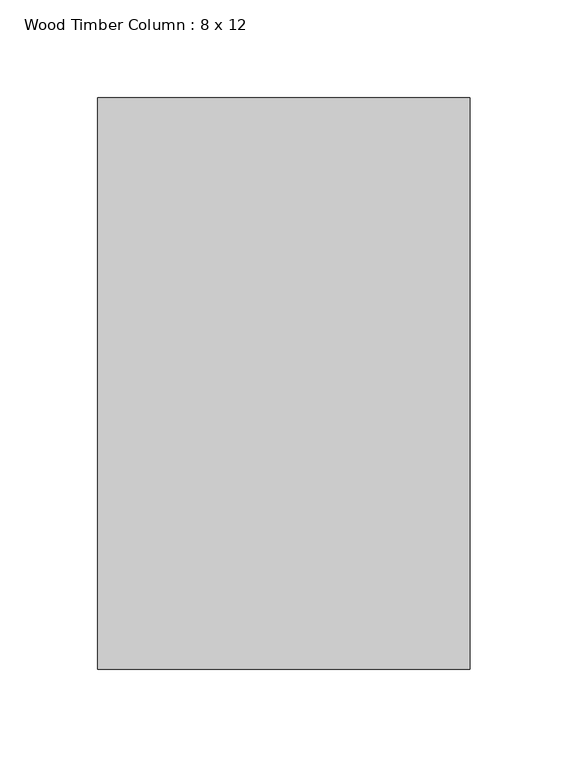
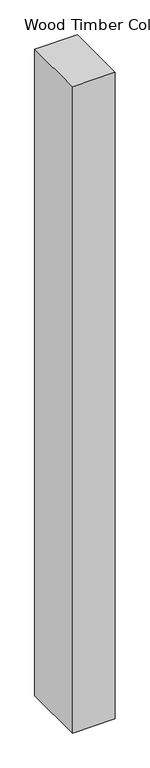
"""IFC4 building model written with IfcOpenShell, lengths in millimetres: column geometry, Wood Timber Column : 8 x 12."""

from ifc_helpers import new_model, si_unit, origin, origin_with_axes, place, context, project, spatial, polyline, outline, extrude, source, transform, mapped, element, save


def wood_timber_column_8_x_12_245a0583(model_context):
    return source(origin(), model_context, "Body", "SweptSolid", [
        extrude(outline(polyline([(95.25, -146.05), (-95.25, -146.05), (-95.25, 146.05), (95.25, 146.05), (95.25, -146.05)])), origin_with_axes(), (0.0, 0.0, 1.0), 3048.0),
    ])


if __name__ == "__main__":
    model = new_model("IFC4")
    model_context = context("Model", 3, world=origin())
    ifc_project = project(units=[si_unit("LENGTHUNIT", "METRE", prefix="MILLI")], contexts=[model_context])
    site = spatial("IfcSite", under=ifc_project)
    building = spatial("IfcBuilding", under=site)
    placement = place(None, origin())
    wood_timber_column_8_x_12_shape = wood_timber_column_8_x_12_245a0583(model_context)
    element("IfcColumn", 1, ObjectType="Wood Timber Column : 8 x 12", at=placement, inside=building, context=model_context, shape_type="MappedRepresentation", body=[
        mapped(wood_timber_column_8_x_12_shape, transform((0.0, 0.0, 0.0), x_axis=(1.0, 0.0, 0.0), y_axis=(0.0, 1.0, 0.0), z_axis=(0.0, 0.0, 1.0))),
    ])
    save(model, "model.ifc")

# Revit data of these elements
# Type "Wood Timber Column : 8 x 12"
#   Assembly Code = "B1010200"
#   Depth = 0' - 11 1/2"
#   Width = 0' - 7 1/2"
#   Material = Softwood, Lumber
# Element 1 (IfcColumn, "Wood Timber Column : 8 x 12")
#   Materials on its faces: "Softwood, Lumber"
# Materials
#   "Softwood, Lumber": class "Wood", colour RGB 223 192 134, transparency 0, Description = "Pinus Echinata", Cost = 0
